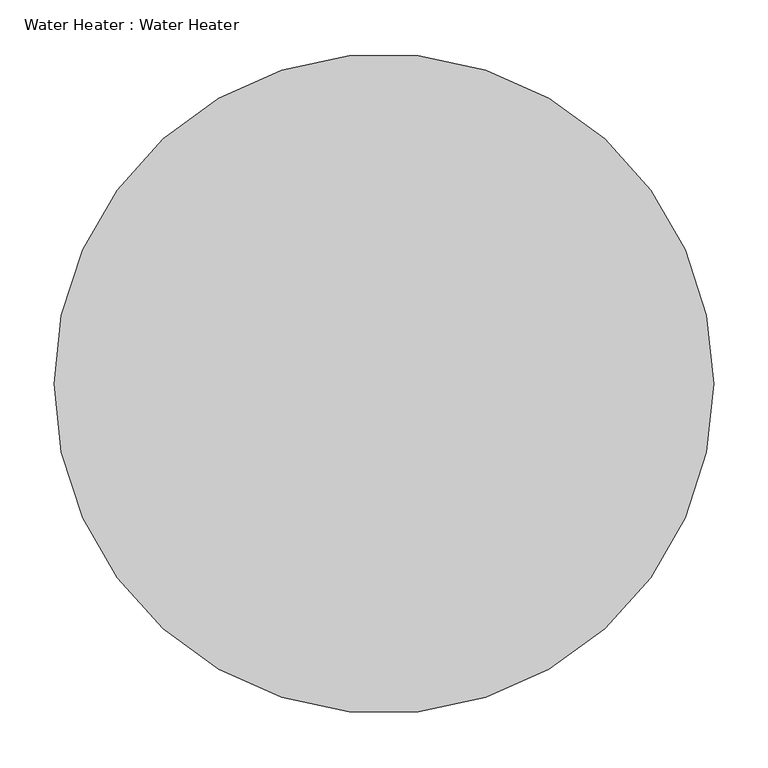
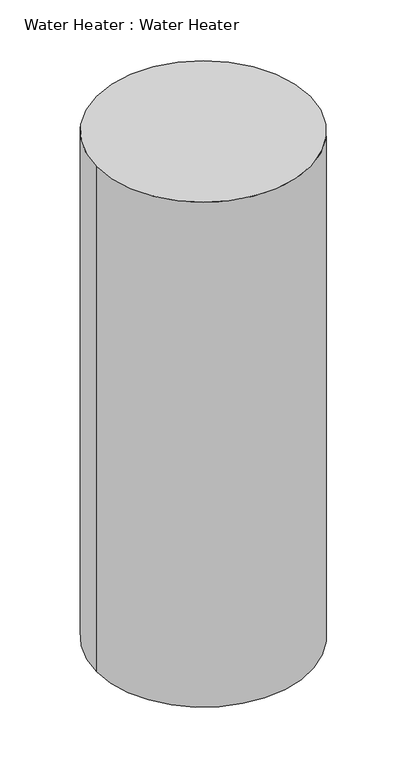
"""IFC4 building model written with IfcOpenShell, lengths in millimetres: flow terminal geometry, Water Heater : Water Heater."""

from ifc_helpers import new_model, si_unit, point, origin, origin_with_axes, origin_2d, place, context, project, spatial, circle_curve, trimmed, segment, composite_curve, outline, extrude, source, transform, mapped, element, save


def water_heater_water_heater_e0cc5f81(model_context):
    return source(origin(), model_context, "Body", "SweptSolid", [
        extrude(outline(composite_curve([segment(trimmed(circle_curve(origin_2d(), 304.8), [point((-304.8, 0.0))], [point((304.8, 0.0))], False, "CARTESIAN"), True, "CONTINUOUS"), segment(trimmed(circle_curve(origin_2d(), 304.8), [point((304.8, 0.0))], [point((-304.8, 0.0))], False, "CARTESIAN"), True, "CONTINUOUS")], self_intersect=False)), origin_with_axes(), (0.0, 0.0, 1.0), 1524.0),
    ])


if __name__ == "__main__":
    model = new_model("IFC4")
    model_context = context("Model", 3, world=origin())
    ifc_project = project(units=[si_unit("LENGTHUNIT", "METRE", prefix="MILLI")], contexts=[model_context])
    site = spatial("IfcSite", under=ifc_project)
    building = spatial("IfcBuilding", under=site)
    placement = place(None, origin())
    water_heater_water_heater_shape = water_heater_water_heater_e0cc5f81(model_context)
    element("IfcFlowTerminal", 1, ObjectType="Water Heater : Water Heater", at=placement, inside=building, context=model_context, shape_type="MappedRepresentation", body=[
        mapped(water_heater_water_heater_shape, transform((0.0, 0.0, 0.0), x_axis=(1.0, 0.0, 0.0), y_axis=(0.0, 1.0, 0.0), z_axis=(0.0, 0.0, 1.0))),
    ])
    save(model, "model.ifc")

# Revit data of these elements
# Type "Water Heater : Water Heater"
#   Label = "WH"
#   Assembly Code = "D2020200"
#   Diameter = 2' - 0"
#   Height = 5' - 0"
#   Default Elevation = 0
